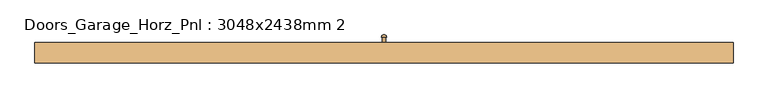
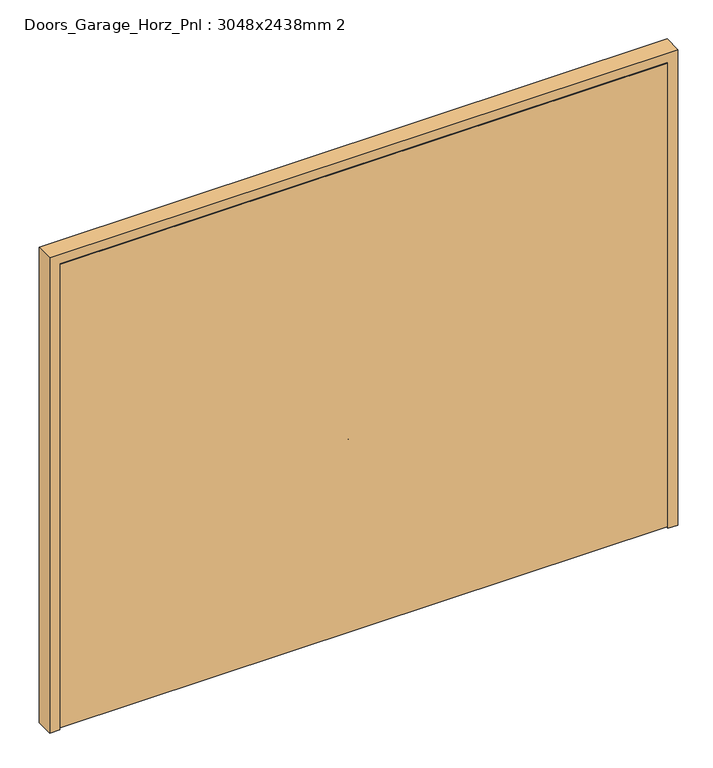
"""IFC4 building model written with IfcOpenShell, lengths in millimetres: door geometry, Doors_Garage_Horz_Pnl : 3048x2438mm 2."""

from ifc_helpers import new_model, si_unit, point, frame, frame_2d, origin, place, context, project, spatial, polyline, circle_curve, ellipse_curve, trimmed, segment, composite_curve, outline, extrude, faceted_brep, source, transform, mapped, element, save
from ifc_brep_helpers import plane_surface, revolved_surface, advanced_brep


def doors_garage_horz_pnl_3048x2438mm_2_abfe55f9(model_context):
    return source(origin(), model_context, "Body", "SolidModel", [
        extrude(outline(composite_curve([segment(trimmed(circle_curve(frame_2d((900.0, 388.5)), 20.0), [point((900.0, 368.5))], [point((900.0, 408.5))], False, "CARTESIAN"), True, "CONTINUOUS"), segment(trimmed(circle_curve(frame_2d((900.0, 388.5)), 20.0), [point((900.0, 408.5))], [point((900.0, 368.5))], False, "CARTESIAN"), True, "CONTINUOUS")], self_intersect=False)), frame((0.0, 80.0, 0.0), z_axis=(0.0, 1.0, 0.0), x_axis=(0.0, 0.0, 1.0)), (0.0, 0.0, 1.0), 3.0),
        advanced_brep(
        [(388.5, 113.0, 843.6641808), (390.3492572, 113.0, 845.2113613), (399.4509795, 113.0, 899.2132014), (390.0, 113.0, 908.6641808), (388.5, 113.0, 908.6641808), (387.0, 113.0, 908.6641808), (377.5490205, 113.0, 899.2132014), (386.6507428, 113.0, 845.2113613)],
        [
            (0, 1, circle_curve(frame((388.1345333, 113.0, 845.979749), z_axis=(0.0, -1.0, 0.0), x_axis=(0.0, 0.0, -1.0)), 2.3442316)),
            (1, 2, circle_curve(frame((234.6997375, 113.0, 899.2132014), z_axis=(0.0, -1.0, 0.0), x_axis=(0.0, 0.0, -1.0)), 164.7512419)),
            (2, 3, circle_curve(frame((390.0, 113.0, 899.2132014), z_axis=(0.0, -1.0, 0.0), x_axis=(0.0, 0.0, -1.0)), 9.4509795)),
            (3, 4),
            (4, 0),
            (4, 5),
            (5, 6, circle_curve(frame((387.0, 113.0, 899.2132014), z_axis=(0.0, -1.0, 0.0), x_axis=(0.0, 0.0, -1.0)), 9.4509795)),
            (6, 7, circle_curve(frame((542.3002625, 113.0, 899.2132014), z_axis=(0.0, -1.0, 0.0), x_axis=(0.0, 0.0, -1.0)), 164.7512419)),
            (7, 0, circle_curve(frame((388.8654667, 113.0, 845.979749), z_axis=(0.0, -1.0, 0.0), x_axis=(0.0, 0.0, -1.0)), 2.3442316)),
            (7, 1, circle_curve(frame((388.5, 113.0, 845.2113613), z_axis=(0.0, 0.0, -1.0), x_axis=(1.0, 0.0, 0.0)), 1.8492572)),
            (6, 2, circle_curve(frame((388.5, 113.0, 899.2132014), z_axis=(0.0, 0.0, -1.0), x_axis=(1.0, 0.0, 0.0)), 10.9509795)),
            (5, 3, circle_curve(frame((388.5, 113.0, 908.6641808), z_axis=(0.0, 0.0, -1.0), x_axis=(1.0, 0.0, 0.0)), 1.5)),
        ],
        [
            plane_surface(frame((388.5, 113.0, 853.0919868), z_axis=(0.0, -1.0, 0.0), x_axis=(1.0, 0.0, 0.0))),
            plane_surface(frame((388.5, 113.0, 853.0919868), z_axis=(0.0, -1.0, 0.0), x_axis=(-1.0, 0.0, 0.0))),
            revolved_surface(trimmed(ellipse_curve(frame((388.1345333, 113.0, 845.979749), z_axis=(0.0, -1.0, 0.0), x_axis=(0.0, 0.0, -1.0)), 2.3442316, 2.3442316), [point((388.5, 113.0, 843.6641808))], [point((390.3492572, 113.0, 845.2113613))], True, "CARTESIAN"), (388.5, 113.0, 853.0919868), (0.0, 0.0, 1.0)),
            revolved_surface(trimmed(ellipse_curve(frame((234.6997375, 113.0, 899.2132014), z_axis=(0.0, -1.0, 0.0), x_axis=(0.0, 0.0, -1.0)), 164.7512419, 164.7512419), [point((390.3492572, 113.0, 845.2113613))], [point((399.4509795, 113.0, 899.2132014))], True, "CARTESIAN"), (388.5, 113.0, 853.0919868), (0.0, 0.0, 1.0)),
            revolved_surface(trimmed(ellipse_curve(frame((390.0, 113.0, 899.2132014), z_axis=(0.0, -1.0, 0.0), x_axis=(0.0, 0.0, -1.0)), 9.4509795, 9.4509795), [point((399.4509795, 113.0, 899.2132014))], [point((390.0, 113.0, 908.6641808))], True, "CARTESIAN"), (388.5, 113.0, 853.0919868), (0.0, 0.0, 1.0)),
            plane_surface(frame((388.5, 113.0, 908.6641808), z_axis=(0.0, 0.0, 1.0), x_axis=(1.0, 0.0, 0.0))),
        ],
        [
            (0, [[1, 2, 3, 4, 5]]),
            (1, [[6, 7, 8, 9, -5]]),
            (2, [[10, -1, -9]]),
            (3, [[11, -2, -10, -8]]),
            (4, [[12, -3, -11, -7]]),
            (5, [[-4, -12, -6]]),
        ],
    ),
        extrude(outline(composite_curve([segment(trimmed(circle_curve(frame_2d((900.0, 388.5)), 7.0), [point((900.0, 395.5))], [point((900.0, 381.5))], False, "CARTESIAN"), True, "CONTINUOUS"), segment(trimmed(circle_curve(frame_2d((900.0, 388.5)), 7.0), [point((900.0, 381.5))], [point((900.0, 395.5))], False, "CARTESIAN"), True, "CONTINUOUS")], self_intersect=False)), frame((0.0, 83.0, 0.0), z_axis=(0.0, 1.0, 0.0), x_axis=(0.0, 0.0, 1.0)), (0.0, 0.0, 1.0), 30.0),
        faceted_brep([(1842.0, 89.3, 0.0), (1912.5, 89.3, 0.0), (1912.5, 0.3, 0.0), (1864.0, 0.3, 0.0), (1864.0, 47.3, 0.0), (1842.0, 47.3, 0.0), (1842.0, 89.3, 2367.9), (-1065.0, 89.3, 2367.9), (-1065.0, 89.3, 0.0), (-1135.5, 89.3, 0.0), (-1135.5, 89.3, 2438.4), (1912.5, 89.3, 2438.4), (1912.5, 0.3, 2438.4), (-1135.5, 0.3, 2438.4), (-1135.5, 0.3, 0.0), (-1087.0, 0.3, 0.0), (-1087.0, 0.3, 2389.9), (1864.0, 0.3, 2389.9), (1864.0, 47.3, 2389.9), (-1087.0, 47.3, 2389.9), (-1087.0, 47.3, 0.0), (-1065.0, 47.3, 0.0), (-1065.0, 47.3, 2367.9), (1842.0, 47.3, 2367.9)], [[[0, 1, 2, 3, 4, 5]], [[1, 0, 6, 7, 8, 9, 10, 11]], [[2, 1, 11, 12]], [[3, 2, 12, 13, 14, 15, 16, 17]], [[4, 3, 17, 18]], [[5, 4, 18, 19, 20, 21, 22, 23]], [[0, 5, 23, 6]], [[7, 22, 21, 8]], [[8, 21, 20, 15, 14, 9]], [[13, 10, 9, 14]], [[19, 16, 15, 20]], [[12, 11, 10, 13]], [[18, 17, 16, 19]], [[6, 23, 22, 7]]]),
        extrude(outline(polyline([(1861.0, 0.3), (-1084.0, 0.3), (-1084.0, 44.3), (1861.0, 44.3), (1861.0, 0.3)])), frame((0.0, 0.0, 10.0), z_axis=(0.0, 0.0, 1.0), x_axis=(1.0, 0.0, 0.0)), (0.0, 0.0, 1.0), 2376.9),
    ])


if __name__ == "__main__":
    model = new_model("IFC4")
    model_context = context("Model", 3, world=origin())
    ifc_project = project(units=[si_unit("LENGTHUNIT", "METRE", prefix="MILLI")], contexts=[model_context])
    site = spatial("IfcSite", under=ifc_project)
    building = spatial("IfcBuilding", under=site)
    placement = place(None, origin())
    doors_garage_horz_pnl_3048x2438mm_2_shape = doors_garage_horz_pnl_3048x2438mm_2_abfe55f9(model_context)
    element("IfcDoor", 1, ObjectType="Doors_Garage_Horz_Pnl : 3048x2438mm 2", at=placement, inside=building, context=model_context, shape_type="MappedRepresentation", body=[
        mapped(doors_garage_horz_pnl_3048x2438mm_2_shape, transform((0.0, 0.0, 0.0), x_axis=(1.0, 0.0, 0.0), y_axis=(0.0, 1.0, 0.0), z_axis=(0.0, 0.0, 1.0))),
    ])
    save(model, "model.ifc")

# Revit data of these elements
# Type "Doors_Garage_Horz_Pnl : 3048x2438mm 2"
#   Type Mark = "20"
#   Type Comments = "External Garage"
#   Operation = "RollingUp"
#   Construction Type Id = "MDOOR"
#   Keynote = "L20"
#   Analytic Construction = "Metal"
#   Wrap Layers (Ext) from Ext = 0' - 4.03543"
#   Wrap Layers (Int) from Ext = 0' - 6.98819"
#   Thickness = 0' - 1.73228"
#   Rough Width = 10' - 0"
#   Rough Height = 8' - 0"
#   O/A Frame Width = 0' - 2.51969"
#   Heat Transfer Coefficient (U) = 0.651978 BTU/(h·ft²·°F)
#   Handle Z Distance = 2' - 11.43307"
#   FrameWidth = 0' - 1.65354"
#   FrameOffset - External = 0' - 0.98425"
#   FrameDepth = 0' - 3.50394"
#   Door Panel Thickness = 0' - 1.73228"
#   Height = 8' - 0"
#   Structural Tolerance = 0' - 0.25591"
#   Tolerance = 0' - 0.11811"
#   Undercut = 0' - 0.3937"
#   Width = 10' - 0"
#   Cavity Closer Width = 0' - 1.9685"
#   Cavity Closer Offset from Ext = 0' - 4.03543"
#   Cavity Closer Depth = 0' - 2.95276"
#   Vis - Ironmongery = yes
#   Vis - Cavity Closers = yes
#   Define Thermal Properties by = 1
#   Function = 1
#   Material Door = Door - Panel
#   Material Frame = Door - Frame/Mullion
#   Material Ironmongery = Door - Handle
#   Visual Light Transmittance = 0
#   Solar Heat Gain Coefficient = 0
#   Wall Closure = (empty or 0)
# Element 1 (IfcDoor, "Doors_Garage_Horz_Pnl : 3048x2438mm 2")
#   Materials on its faces: "Door - Handle", "Door - Frame/Mullion", "Door - Panel"
# Materials
#   "Door - Panel": class "Wood", colour RGB 210 159 95, transparency 0, Cost = 0
#   "Door - Frame/Mullion": class "Wood", colour RGB 212 179 113, transparency 0
#   "Door - Handle": colour RGB 246 240 166, transparency 0
